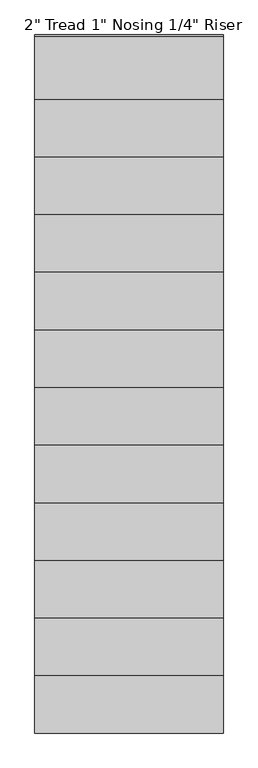
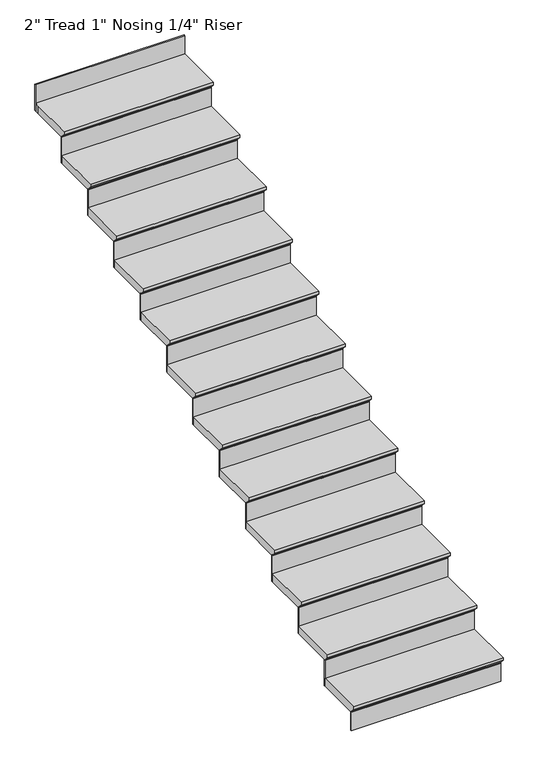
"""IFC4 building model written with IfcOpenShell, lengths in millimetres: stair flight geometry."""

from ifc_helpers import new_model, si_unit, origin, place, context, project, spatial, faceted_brep, source, transform, mapped, element, save


def stair_flight_d970984e(model_context):
    return source(origin(), model_context, "Body", "Brep", [
        faceted_brep([(-2703.0415084, 19841.9216096, 46720.9005799), (-2703.0415084, 19841.9216096, 46739.9505799), (-3617.4415084, 19841.9216096, 46739.9505799), (-3617.4415084, 19841.9216096, 46720.9005799), (-2703.0415084, 19867.3216096, 46695.5005799), (-3617.4415084, 19867.3216096, 46695.5005799), (-2703.0415084, 20146.7216096, 46739.9505799), (-3617.4415084, 20146.7216096, 46739.9505799), (-3617.4415084, 19867.3216096, 46689.1505799), (-3617.4415084, 20146.7216096, 46689.1505799), (-2703.0415084, 20146.7216096, 46689.1505799), (-2703.0415084, 19867.3216096, 46689.1505799)], [[[0, 1, 2, 3]], [[4, 0, 3, 5]], [[2, 1, 6, 7]], [[8, 9, 10, 11]], [[2, 7, 9, 8, 5, 3]], [[8, 11, 4, 5]], [[6, 1, 0, 4, 11, 10]], [[7, 6, 10, 9]]]),
        faceted_brep([(-2703.0415084, 19867.3216096, 46689.1505799), (-2703.0415084, 19867.3216096, 46570.6172466), (-2703.0415084, 19873.6716096, 46570.6172466), (-2703.0415084, 19873.6716096, 46689.1505799), (-3617.4415084, 19867.3216096, 46689.1505799), (-3617.4415084, 19873.6716096, 46689.1505799), (-3617.4415084, 19873.6716096, 46570.6172466), (-3617.4415084, 19867.3216096, 46570.6172466)], [[[0, 1, 2, 3]], [[4, 5, 6, 7]], [[1, 0, 4, 7]], [[2, 1, 7, 6]], [[3, 2, 6, 5]], [[0, 3, 5, 4]]]),
        faceted_brep([(-2703.0415084, 20146.7216096, 46858.4839133), (-2703.0415084, 20146.7216096, 46689.1505799), (-2703.0415084, 20153.0716096, 46689.1505799), (-2703.0415084, 20153.0716096, 46858.4839133), (-3617.4415084, 20146.7216096, 46858.4839133), (-3617.4415084, 20153.0716096, 46858.4839133), (-3617.4415084, 20153.0716096, 46689.1505799), (-3617.4415084, 20146.7216096, 46689.1505799)], [[[0, 1, 2, 3]], [[4, 5, 6, 7]], [[1, 0, 4, 7]], [[2, 1, 7, 6]], [[3, 2, 6, 5]], [[0, 3, 5, 4]]]),
        faceted_brep([(-3617.4415084, 20121.3216096, 46909.2839133), (-2703.0415084, 20121.3216096, 46909.2839133), (-2703.0415084, 20426.1216096, 46909.2839133), (-3617.4415084, 20426.1216096, 46909.2839133), (-3617.4415084, 20146.7216096, 46858.4839133), (-3617.4415084, 20426.1216096, 46858.4839133), (-2703.0415084, 20426.1216096, 46858.4839133), (-2703.0415084, 20146.7216096, 46858.4839133), (-3617.4415084, 20146.7216096, 46864.8339133), (-3617.4415084, 20121.3216096, 46890.2339133), (-2703.0415084, 20146.7216096, 46864.8339133), (-2703.0415084, 20121.3216096, 46890.2339133)], [[[0, 1, 2, 3]], [[4, 5, 6, 7]], [[0, 3, 5, 4, 8, 9]], [[4, 7, 10, 8]], [[2, 1, 11, 10, 7, 6]], [[3, 2, 6, 5]], [[11, 1, 0, 9]], [[10, 11, 9, 8]]]),
        faceted_brep([(-2703.0415084, 20426.1216096, 47027.8172466), (-2703.0415084, 20426.1216096, 46858.4839133), (-2703.0415084, 20432.4716096, 46858.4839133), (-2703.0415084, 20432.4716096, 47027.8172466), (-3617.4415084, 20426.1216096, 47027.8172466), (-3617.4415084, 20432.4716096, 47027.8172466), (-3617.4415084, 20432.4716096, 46858.4839133), (-3617.4415084, 20426.1216096, 46858.4839133)], [[[0, 1, 2, 3]], [[4, 5, 6, 7]], [[1, 0, 4, 7]], [[2, 1, 7, 6]], [[3, 2, 6, 5]], [[0, 3, 5, 4]]]),
        faceted_brep([(-3617.4415084, 20400.7216096, 47078.6172466), (-2703.0415084, 20400.7216096, 47078.6172466), (-2703.0415084, 20705.5216096, 47078.6172466), (-3617.4415084, 20705.5216096, 47078.6172466), (-3617.4415084, 20426.1216096, 47027.8172466), (-3617.4415084, 20705.5216096, 47027.8172466), (-2703.0415084, 20705.5216096, 47027.8172466), (-2703.0415084, 20426.1216096, 47027.8172466), (-3617.4415084, 20426.1216096, 47034.1672466), (-3617.4415084, 20400.7216096, 47059.5672466), (-2703.0415084, 20426.1216096, 47034.1672466), (-2703.0415084, 20400.7216096, 47059.5672466)], [[[0, 1, 2, 3]], [[4, 5, 6, 7]], [[0, 3, 5, 4, 8, 9]], [[4, 7, 10, 8]], [[2, 1, 11, 10, 7, 6]], [[3, 2, 6, 5]], [[11, 1, 0, 9]], [[10, 11, 9, 8]]]),
        faceted_brep([(-2703.0415084, 20705.5216096, 47197.1505799), (-2703.0415084, 20705.5216096, 47027.8172466), (-2703.0415084, 20711.8716096, 47027.8172466), (-2703.0415084, 20711.8716096, 47197.1505799), (-3617.4415084, 20705.5216096, 47197.1505799), (-3617.4415084, 20711.8716096, 47197.1505799), (-3617.4415084, 20711.8716096, 47027.8172466), (-3617.4415084, 20705.5216096, 47027.8172466)], [[[0, 1, 2, 3]], [[4, 5, 6, 7]], [[1, 0, 4, 7]], [[2, 1, 7, 6]], [[3, 2, 6, 5]], [[0, 3, 5, 4]]]),
        faceted_brep([(-3617.4415084, 20680.1216096, 47247.9505799), (-2703.0415084, 20680.1216096, 47247.9505799), (-2703.0415084, 20984.9216096, 47247.9505799), (-3617.4415084, 20984.9216096, 47247.9505799), (-3617.4415084, 20705.5216096, 47197.1505799), (-3617.4415084, 20984.9216096, 47197.1505799), (-2703.0415084, 20984.9216096, 47197.1505799), (-2703.0415084, 20705.5216096, 47197.1505799), (-3617.4415084, 20705.5216096, 47203.5005799), (-3617.4415084, 20680.1216096, 47228.9005799), (-2703.0415084, 20705.5216096, 47203.5005799), (-2703.0415084, 20680.1216096, 47228.9005799)], [[[0, 1, 2, 3]], [[4, 5, 6, 7]], [[0, 3, 5, 4, 8, 9]], [[4, 7, 10, 8]], [[2, 1, 11, 10, 7, 6]], [[3, 2, 6, 5]], [[11, 1, 0, 9]], [[10, 11, 9, 8]]]),
        faceted_brep([(-2703.0415084, 20984.9216096, 47366.4839133), (-2703.0415084, 20984.9216096, 47197.1505799), (-2703.0415084, 20991.2716096, 47197.1505799), (-2703.0415084, 20991.2716096, 47366.4839133), (-3617.4415084, 20984.9216096, 47366.4839133), (-3617.4415084, 20991.2716096, 47366.4839133), (-3617.4415084, 20991.2716096, 47197.1505799), (-3617.4415084, 20984.9216096, 47197.1505799)], [[[0, 1, 2, 3]], [[4, 5, 6, 7]], [[1, 0, 4, 7]], [[2, 1, 7, 6]], [[3, 2, 6, 5]], [[0, 3, 5, 4]]]),
        faceted_brep([(-3617.4415084, 20959.5216096, 47417.2839133), (-2703.0415084, 20959.5216096, 47417.2839133), (-2703.0415084, 21264.3216096, 47417.2839133), (-3617.4415084, 21264.3216096, 47417.2839133), (-3617.4415084, 20984.9216096, 47366.4839133), (-3617.4415084, 21264.3216096, 47366.4839133), (-2703.0415084, 21264.3216096, 47366.4839133), (-2703.0415084, 20984.9216096, 47366.4839133), (-3617.4415084, 20984.9216096, 47372.8339133), (-3617.4415084, 20959.5216096, 47398.2339133), (-2703.0415084, 20984.9216096, 47372.8339133), (-2703.0415084, 20959.5216096, 47398.2339133)], [[[0, 1, 2, 3]], [[4, 5, 6, 7]], [[0, 3, 5, 4, 8, 9]], [[4, 7, 10, 8]], [[2, 1, 11, 10, 7, 6]], [[3, 2, 6, 5]], [[11, 1, 0, 9]], [[10, 11, 9, 8]]]),
        faceted_brep([(-2703.0415084, 21264.3216096, 47535.8172466), (-2703.0415084, 21264.3216096, 47366.4839133), (-2703.0415084, 21270.6716096, 47366.4839133), (-2703.0415084, 21270.6716096, 47535.8172466), (-3617.4415084, 21264.3216096, 47535.8172466), (-3617.4415084, 21270.6716096, 47535.8172466), (-3617.4415084, 21270.6716096, 47366.4839133), (-3617.4415084, 21264.3216096, 47366.4839133)], [[[0, 1, 2, 3]], [[4, 5, 6, 7]], [[1, 0, 4, 7]], [[2, 1, 7, 6]], [[3, 2, 6, 5]], [[0, 3, 5, 4]]]),
        faceted_brep([(-3617.4415084, 21238.9216096, 47586.6172466), (-2703.0415084, 21238.9216096, 47586.6172466), (-2703.0415084, 21543.7216096, 47586.6172466), (-3617.4415084, 21543.7216096, 47586.6172466), (-3617.4415084, 21264.3216096, 47535.8172466), (-3617.4415084, 21543.7216096, 47535.8172466), (-2703.0415084, 21543.7216096, 47535.8172466), (-2703.0415084, 21264.3216096, 47535.8172466), (-3617.4415084, 21264.3216096, 47542.1672466), (-3617.4415084, 21238.9216096, 47567.5672466), (-2703.0415084, 21264.3216096, 47542.1672466), (-2703.0415084, 21238.9216096, 47567.5672466)], [[[0, 1, 2, 3]], [[4, 5, 6, 7]], [[0, 3, 5, 4, 8, 9]], [[4, 7, 10, 8]], [[2, 1, 11, 10, 7, 6]], [[3, 2, 6, 5]], [[11, 1, 0, 9]], [[10, 11, 9, 8]]]),
        faceted_brep([(-2703.0415084, 21543.7216096, 47705.1505799), (-2703.0415084, 21543.7216096, 47535.8172466), (-2703.0415084, 21550.0716096, 47535.8172466), (-2703.0415084, 21550.0716096, 47705.1505799), (-3617.4415084, 21543.7216096, 47705.1505799), (-3617.4415084, 21550.0716096, 47705.1505799), (-3617.4415084, 21550.0716096, 47535.8172466), (-3617.4415084, 21543.7216096, 47535.8172466)], [[[0, 1, 2, 3]], [[4, 5, 6, 7]], [[1, 0, 4, 7]], [[2, 1, 7, 6]], [[3, 2, 6, 5]], [[0, 3, 5, 4]]]),
        faceted_brep([(-3617.4415084, 21518.3216096, 47755.9505799), (-2703.0415084, 21518.3216096, 47755.9505799), (-2703.0415084, 21823.1216096, 47755.9505799), (-3617.4415084, 21823.1216096, 47755.9505799), (-3617.4415084, 21543.7216096, 47705.1505799), (-3617.4415084, 21823.1216096, 47705.1505799), (-2703.0415084, 21823.1216096, 47705.1505799), (-2703.0415084, 21543.7216096, 47705.1505799), (-3617.4415084, 21543.7216096, 47711.5005799), (-3617.4415084, 21518.3216096, 47736.9005799), (-2703.0415084, 21543.7216096, 47711.5005799), (-2703.0415084, 21518.3216096, 47736.9005799)], [[[0, 1, 2, 3]], [[4, 5, 6, 7]], [[0, 3, 5, 4, 8, 9]], [[4, 7, 10, 8]], [[2, 1, 11, 10, 7, 6]], [[3, 2, 6, 5]], [[11, 1, 0, 9]], [[10, 11, 9, 8]]]),
        faceted_brep([(-2703.0415084, 21823.1216096, 47874.4839133), (-2703.0415084, 21823.1216096, 47705.1505799), (-2703.0415084, 21829.4716096, 47705.1505799), (-2703.0415084, 21829.4716096, 47874.4839133), (-3617.4415084, 21823.1216096, 47874.4839133), (-3617.4415084, 21829.4716096, 47874.4839133), (-3617.4415084, 21829.4716096, 47705.1505799), (-3617.4415084, 21823.1216096, 47705.1505799)], [[[0, 1, 2, 3]], [[4, 5, 6, 7]], [[1, 0, 4, 7]], [[2, 1, 7, 6]], [[3, 2, 6, 5]], [[0, 3, 5, 4]]]),
        faceted_brep([(-3617.4415084, 21797.7216096, 47925.2839133), (-2703.0415084, 21797.7216096, 47925.2839133), (-2703.0415084, 22102.5216096, 47925.2839133), (-3617.4415084, 22102.5216096, 47925.2839133), (-3617.4415084, 21823.1216096, 47874.4839133), (-3617.4415084, 22102.5216096, 47874.4839133), (-2703.0415084, 22102.5216096, 47874.4839133), (-2703.0415084, 21823.1216096, 47874.4839133), (-3617.4415084, 21823.1216096, 47880.8339133), (-3617.4415084, 21797.7216096, 47906.2339133), (-2703.0415084, 21823.1216096, 47880.8339133), (-2703.0415084, 21797.7216096, 47906.2339133)], [[[0, 1, 2, 3]], [[4, 5, 6, 7]], [[0, 3, 5, 4, 8, 9]], [[4, 7, 10, 8]], [[2, 1, 11, 10, 7, 6]], [[3, 2, 6, 5]], [[11, 1, 0, 9]], [[10, 11, 9, 8]]]),
        faceted_brep([(-2703.0415084, 22102.5216096, 48043.8172466), (-2703.0415084, 22102.5216096, 47874.4839133), (-2703.0415084, 22108.8716096, 47874.4839133), (-2703.0415084, 22108.8716096, 48043.8172466), (-3617.4415084, 22102.5216096, 48043.8172466), (-3617.4415084, 22108.8716096, 48043.8172466), (-3617.4415084, 22108.8716096, 47874.4839133), (-3617.4415084, 22102.5216096, 47874.4839133)], [[[0, 1, 2, 3]], [[4, 5, 6, 7]], [[1, 0, 4, 7]], [[2, 1, 7, 6]], [[3, 2, 6, 5]], [[0, 3, 5, 4]]]),
        faceted_brep([(-3617.4415084, 22077.1216096, 48094.6172466), (-2703.0415084, 22077.1216096, 48094.6172466), (-2703.0415084, 22381.9216096, 48094.6172466), (-3617.4415084, 22381.9216096, 48094.6172466), (-3617.4415084, 22102.5216096, 48043.8172466), (-3617.4415084, 22381.9216096, 48043.8172466), (-2703.0415084, 22381.9216096, 48043.8172466), (-2703.0415084, 22102.5216096, 48043.8172466), (-3617.4415084, 22102.5216096, 48050.1672466), (-3617.4415084, 22077.1216096, 48075.5672466), (-2703.0415084, 22102.5216096, 48050.1672466), (-2703.0415084, 22077.1216096, 48075.5672466)], [[[0, 1, 2, 3]], [[4, 5, 6, 7]], [[0, 3, 5, 4, 8, 9]], [[4, 7, 10, 8]], [[2, 1, 11, 10, 7, 6]], [[3, 2, 6, 5]], [[11, 1, 0, 9]], [[10, 11, 9, 8]]]),
        faceted_brep([(-2703.0415084, 22381.9216096, 48213.1505799), (-2703.0415084, 22381.9216096, 48043.8172466), (-2703.0415084, 22388.2716096, 48043.8172466), (-2703.0415084, 22388.2716096, 48213.1505799), (-3617.4415084, 22381.9216096, 48213.1505799), (-3617.4415084, 22388.2716096, 48213.1505799), (-3617.4415084, 22388.2716096, 48043.8172466), (-3617.4415084, 22381.9216096, 48043.8172466)], [[[0, 1, 2, 3]], [[4, 5, 6, 7]], [[1, 0, 4, 7]], [[2, 1, 7, 6]], [[3, 2, 6, 5]], [[0, 3, 5, 4]]]),
        faceted_brep([(-3617.4415084, 22356.5216096, 48263.9505799), (-2703.0415084, 22356.5216096, 48263.9505799), (-2703.0415084, 22661.3216096, 48263.9505799), (-3617.4415084, 22661.3216096, 48263.9505799), (-3617.4415084, 22381.9216096, 48213.1505799), (-3617.4415084, 22661.3216096, 48213.1505799), (-2703.0415084, 22661.3216096, 48213.1505799), (-2703.0415084, 22381.9216096, 48213.1505799), (-3617.4415084, 22381.9216096, 48219.5005799), (-3617.4415084, 22356.5216096, 48244.9005799), (-2703.0415084, 22381.9216096, 48219.5005799), (-2703.0415084, 22356.5216096, 48244.9005799)], [[[0, 1, 2, 3]], [[4, 5, 6, 7]], [[0, 3, 5, 4, 8, 9]], [[4, 7, 10, 8]], [[2, 1, 11, 10, 7, 6]], [[3, 2, 6, 5]], [[11, 1, 0, 9]], [[10, 11, 9, 8]]]),
        faceted_brep([(-2703.0415084, 22661.3216096, 48382.4839133), (-2703.0415084, 22661.3216096, 48213.1505799), (-2703.0415084, 22667.6716096, 48213.1505799), (-2703.0415084, 22667.6716096, 48382.4839133), (-3617.4415084, 22661.3216096, 48382.4839133), (-3617.4415084, 22667.6716096, 48382.4839133), (-3617.4415084, 22667.6716096, 48213.1505799), (-3617.4415084, 22661.3216096, 48213.1505799)], [[[0, 1, 2, 3]], [[4, 5, 6, 7]], [[1, 0, 4, 7]], [[2, 1, 7, 6]], [[3, 2, 6, 5]], [[0, 3, 5, 4]]]),
        faceted_brep([(-3617.4415084, 22635.9216096, 48433.2839133), (-2703.0415084, 22635.9216096, 48433.2839133), (-2703.0415084, 22940.7216096, 48433.2839133), (-3617.4415084, 22940.7216096, 48433.2839133), (-3617.4415084, 22661.3216096, 48382.4839133), (-3617.4415084, 22940.7216096, 48382.4839133), (-2703.0415084, 22940.7216096, 48382.4839133), (-2703.0415084, 22661.3216096, 48382.4839133), (-3617.4415084, 22661.3216096, 48388.8339133), (-3617.4415084, 22635.9216096, 48414.2339133), (-2703.0415084, 22661.3216096, 48388.8339133), (-2703.0415084, 22635.9216096, 48414.2339133)], [[[0, 1, 2, 3]], [[4, 5, 6, 7]], [[0, 3, 5, 4, 8, 9]], [[4, 7, 10, 8]], [[2, 1, 11, 10, 7, 6]], [[3, 2, 6, 5]], [[11, 1, 0, 9]], [[10, 11, 9, 8]]]),
        faceted_brep([(-2703.0415084, 23220.1216096, 48721.1505799), (-2703.0415084, 23220.1216096, 48551.8172466), (-2703.0415084, 23226.4716096, 48551.8172466), (-2703.0415084, 23226.4716096, 48721.1505799), (-3617.4415084, 23220.1216096, 48721.1505799), (-3617.4415084, 23226.4716096, 48721.1505799), (-3617.4415084, 23226.4716096, 48551.8172466), (-3617.4415084, 23220.1216096, 48551.8172466)], [[[0, 1, 2, 3]], [[4, 5, 6, 7]], [[1, 0, 4, 7]], [[2, 1, 7, 6]], [[3, 2, 6, 5]], [[0, 3, 5, 4]]]),
        faceted_brep([(-2703.0415084, 22940.7216096, 48551.8172466), (-2703.0415084, 22940.7216096, 48382.4839133), (-2703.0415084, 22947.0716096, 48382.4839133), (-2703.0415084, 22947.0716096, 48551.8172466), (-3617.4415084, 22940.7216096, 48551.8172466), (-3617.4415084, 22947.0716096, 48551.8172466), (-3617.4415084, 22947.0716096, 48382.4839133), (-3617.4415084, 22940.7216096, 48382.4839133)], [[[0, 1, 2, 3]], [[4, 5, 6, 7]], [[1, 0, 4, 7]], [[2, 1, 7, 6]], [[3, 2, 6, 5]], [[0, 3, 5, 4]]]),
        faceted_brep([(-3617.4415084, 23220.1216096, 48602.6172466), (-3617.4415084, 23194.7216096, 48602.6172466), (-3617.4415084, 22915.3216096, 48602.6172466), (-2703.0415084, 22915.3216096, 48602.6172466), (-2703.0415084, 23220.1216096, 48602.6172466), (-3617.4415084, 23194.7216096, 48551.8172466), (-3617.4415084, 23220.1216096, 48551.8172466), (-2703.0415084, 23220.1216096, 48551.8172466), (-2703.0415084, 22940.7216096, 48551.8172466), (-3617.4415084, 22940.7216096, 48551.8172466), (-3617.4415084, 22940.7216096, 48558.1672466), (-3617.4415084, 22915.3216096, 48583.5672466), (-2703.0415084, 22940.7216096, 48558.1672466), (-2703.0415084, 22915.3216096, 48583.5672466)], [[[0, 1, 2, 3, 4]], [[5, 6, 7, 8, 9]], [[1, 0, 6, 5]], [[2, 1, 5, 9, 10, 11]], [[9, 8, 12, 10]], [[4, 3, 13, 12, 8, 7]], [[0, 4, 7, 6]], [[13, 3, 2, 11]], [[12, 13, 11, 10]]]),
    ])


if __name__ == "__main__":
    model = new_model("IFC4")
    model_context = context("Model", 3, world=origin())
    ifc_project = project(units=[si_unit("LENGTHUNIT", "METRE", prefix="MILLI")], contexts=[model_context])
    site = spatial("IfcSite", under=ifc_project)
    building = spatial("IfcBuilding", under=site)
    placement = place(None, origin())
    stair_flight_shape = stair_flight_d970984e(model_context)
    element("IfcStairFlight", 1, ObjectType="2\" Tread 1\" Nosing 1/4\" Riser", at=placement, inside=building, context=model_context, shape_type="MappedRepresentation", body=[
        mapped(stair_flight_shape, transform((0.0, 0.0, 0.0), x_axis=(1.0, 0.0, 0.0), y_axis=(0.0, 1.0, 0.0), z_axis=(0.0, 0.0, 1.0))),
    ])
    save(model, "model.ifc")
